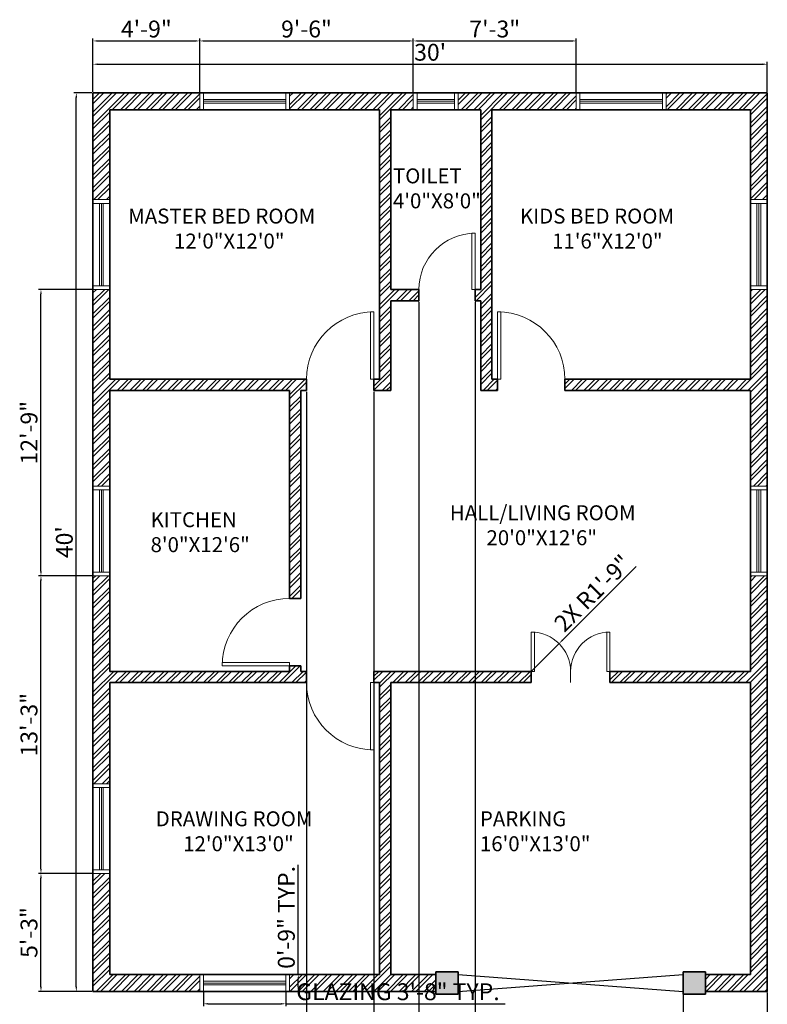
# Model space of a CAD drawing. Units: inches. Extents: x 2639 to 6021, y 292 to 2009.
# Tile 4 of 6: x 2697 to 3096, y 1243 to 1768. Entities that reach past the tile are written whole.
import ezdxf

# ---------------------------------------------------------------- set-up
doc = ezdxf.new("R2010")
doc.units = ezdxf.units.IN
for name, color, linetype, lineweight in [('A-ANNO-DIMS', 2, 'Continuous', 18), ('A-AREA-IDEN', 7, 'Continuous', 18), ('A-COLS', 7, 'Continuous', 35), ('A-DOOR', 3, 'Continuous', 20), ('A-DOOR-GATE', 3, 'Continuous', 25), ('A-GLAZ', 4, 'Continuous', 18), ('A-WALL', 7, 'Continuous', 35)]:
    doc.layers.add(name, color=color, linetype=linetype, lineweight=lineweight)
doc.layers.add('A-COLS-PATT', color=251, linetype='Continuous', lineweight=13, true_color=0x636466)
doc.layers.add('A-WALL-PATT', color=251, linetype='Continuous', lineweight=13, true_color=0x636466)
doc.styles.get("Standard").update_dxf_attribs({"font": 'arial.ttf'})
doc.dimstyles.new('ISO-25', dxfattribs={"dimtxt": 9, "dimasz": 2.5, "dimexe": 1.25, "dimexo": 0.625, "dimtad": 1, "dimdec": 1, "dimlunit": 3, "dimtxsty": 'Standard', "dimcen": 2.5, "dimadec": 0, "dimazin": 0, "dimtfac": 1, "dimtdec": 1, "dimtmove": 0, "dimatfit": 3, "dimfxl": 1, "dimarcsym": 0})

# ---------------------------------------------------------------- blocks, each defined once
blk = doc.blocks.new('*U2')
for p, q in [((0, 0), (0, -6)), ((30, 0), (30, -6))]:
    blk.add_line(p, q)
blk.add_lwpolyline([(0, 0), (0, 30), (1.75, 30), (1.75, 0)], close=True)
blk.add_arc((0, 0), 30, 0, 90)
blk = doc.blocks.new('*U3')
for p, q in [((0, 0), (0, -6)), ((36, 0), (36, -6))]:
    blk.add_line(p, q)
blk.add_lwpolyline([(0, 0), (0, 36), (1.75, 36), (1.75, 0)], close=True)
blk.add_arc((0, 0), 36, 0, 90)
blk = doc.blocks.new('1')
for p, q in [((0, 6), (0, 0)), ((21, 6), (21, 0)), ((21, 6), (21, 0)), ((42, 6), (42, 0))]:
    blk.add_line(p, q)
for points in [[(0, 6), (0, 27), (1.75, 27), (1.75, 6)], [(42, 6), (42, 27), (40.25, 27), (40.25, 6)]]:
    blk.add_lwpolyline(points, close=True)
for centre, start, end in [((0, 6), 0, 90), ((42, 6), 90, 180)]:
    blk.add_arc(centre, 21, start, end)
blk = doc.blocks.new('*D5')
at = {"layer": 'A-ANNO-DIMS', "color": 0, "lineweight": -2, "transparency": 16777216}
for p, q in [((2735.48, 1729.38), (2725.97, 1729.38)), ((2727.22, 1251.88), (2727.22, 1726.88)), ((2735.48, 1249.38), (2725.97, 1249.38))]:
    blk.add_line(p, q, dxfattribs=at)
at = {"layer": 'A-ANNO-DIMS', "color": 0, "transparency": 16777216}
for points in [[(2726.81, 1726.88), (2727.64, 1726.88), (2727.22, 1729.38)], [(2726.81, 1251.88), (2727.64, 1251.88), (2727.22, 1249.38)]]:
    blk.add_solid(points, dxfattribs=at)
at = {"layer": 'Defpoints', "color": 0, "transparency": 16777216}
for p in [(2727.22, 1729.38), (2736.11, 1729.38), (2736.11, 1249.38)]:
    blk.add_point(p, dxfattribs=at)
at = {"layer": 'A-ANNO-DIMS', "color": 0, "transparency": 16777216, "insert": (2722, 1489.38), "char_height": 9, "attachment_point": 5, "rotation": 90}
blk.add_mtext("40'", dxfattribs=at)
blk = doc.blocks.new('*D6')
at = {"layer": 'A-ANNO-DIMS', "color": 0, "lineweight": -2, "transparency": 16777216}
for p, q in [((2736.11, 1730.01), (2736.11, 1745.96)), ((2738.61, 1744.71), (3093.61, 1744.71)), ((3096.11, 1730.01), (3096.11, 1745.96))]:
    blk.add_line(p, q, dxfattribs=at)
at = {"layer": 'A-ANNO-DIMS', "color": 0, "transparency": 16777216}
for points in [[(2738.61, 1745.12), (2738.61, 1744.29), (2736.11, 1744.71)], [(3093.61, 1745.12), (3093.61, 1744.29), (3096.11, 1744.71)]]:
    blk.add_solid(points, dxfattribs=at)
at = {"layer": 'Defpoints', "color": 0, "transparency": 16777216}
for p in [(3096.11, 1744.71), (2736.11, 1729.38), (3096.11, 1729.38)]:
    blk.add_point(p, dxfattribs=at)
at = {"layer": 'A-ANNO-DIMS', "color": 0, "transparency": 16777216, "insert": (2916.11, 1749.93), "char_height": 9, "attachment_point": 5}
blk.add_mtext("30'", dxfattribs=at)
blk = doc.blocks.new('WINDOW-PLAN-48IN')
for p, q in [((0, 9), (0, 0)), ((0, 5.5), (44, 5.5)), ((44, 9), (44, 0)), ((0, 4.5), (44, 4.5)), ((0, 3.5), (44, 3.5))]:
    blk.add_line(p, q)
blk = doc.blocks.new('WINDOW-PLAN-24IN')
for p, q in [((0, 0), (0, 9)), ((0, 5.5), (20, 5.5)), ((20, 0), (20, 9)), ((0, 4.5), (20, 4.5)), ((0, 3.5), (20, 3.5))]:
    blk.add_line(p, q)
blk = doc.blocks.new('GATE-PLAN-10FT')
for p, q in [((0, 9), (120, 0)), ((0, 0), (120, 9))]:
    blk.add_line(p, q)
blk = doc.blocks.new('*D32')
at = {"layer": 'A-ANNO-DIMS', "color": 0, "lineweight": -2, "transparency": 16777216}
for p, q in [((2795.11, 1248.76), (2795.11, 1241.53)), ((2839.11, 1248.76), (2839.11, 1241.53)), ((2797.61, 1242.78), (2836.61, 1242.78)), ((2839.11, 1242.78), (2956.25, 1242.78))]:
    blk.add_line(p, q, dxfattribs=at)
at = {"layer": 'A-ANNO-DIMS', "color": 0, "transparency": 16777216}
for points in [[(2797.61, 1243.2), (2797.61, 1242.37), (2795.11, 1242.78)], [(2836.61, 1243.2), (2836.61, 1242.37), (2839.11, 1242.78)]]:
    blk.add_solid(points, dxfattribs=at)
at = {"layer": 'Defpoints', "color": 0, "transparency": 16777216}
for p in [(2795.11, 1249.38), (2839.11, 1249.38), (2839.11, 1242.78)]:
    blk.add_point(p, dxfattribs=at)
at = {"layer": 'A-ANNO-DIMS', "color": 0, "transparency": 16777216, "insert": (2898.93, 1248.07), "char_height": 9, "attachment_point": 5}
blk.add_mtext('GLAZING 3\'-8" TYP.', dxfattribs=at)
blk = doc.blocks.new('*D33')
at = {"layer": 'A-ANNO-DIMS', "color": 0, "lineweight": -2, "transparency": 16777216}
for p, q in [((2845.71, 1258.38), (2845.71, 1316.99)), ((2839.73, 1258.38), (2846.96, 1258.38)), ((2845.71, 1251.88), (2845.71, 1255.88)), ((2839.73, 1249.38), (2846.96, 1249.38))]:
    blk.add_line(p, q, dxfattribs=at)
at = {"layer": 'A-ANNO-DIMS', "color": 0, "transparency": 16777216}
for points in [[(2845.29, 1255.88), (2846.12, 1255.88), (2845.71, 1258.38)], [(2845.29, 1251.88), (2846.12, 1251.88), (2845.71, 1249.38)]]:
    blk.add_solid(points, dxfattribs=at)
at = {"layer": 'Defpoints', "color": 0, "transparency": 16777216}
for p in [(2839.11, 1258.38), (2845.71, 1258.38), (2839.11, 1249.38)]:
    blk.add_point(p, dxfattribs=at)
at = {"layer": 'A-ANNO-DIMS', "color": 0, "transparency": 16777216, "insert": (2840.49, 1288.94), "char_height": 9, "attachment_point": 5, "rotation": 90}
blk.add_mtext('0\'-9" TYP.', dxfattribs=at)
blk = doc.blocks.new('*D54')
at = {"layer": 'A-ANNO-DIMS', "color": 0, "lineweight": -2, "transparency": 16777216}
for p, q in [((2850.11, 1569.76), (2850.11, 1218.88)), ((2886.11, 1569.76), (2886.11, 1218.88)), ((2852.61, 1220.13), (2883.61, 1220.13))]:
    blk.add_line(p, q, dxfattribs=at)
at = {"layer": 'A-ANNO-DIMS', "color": 0, "transparency": 16777216}
for points in [[(2852.61, 1220.55), (2852.61, 1219.72), (2850.11, 1220.13)], [(2883.61, 1220.55), (2883.61, 1219.72), (2886.11, 1220.13)]]:
    blk.add_solid(points, dxfattribs=at)
at = {"layer": 'Defpoints', "color": 0, "transparency": 16777216}
for p in [(2850.11, 1570.38), (2886.11, 1570.38), (2886.11, 1220.13)]:
    blk.add_point(p, dxfattribs=at)
at = {"layer": 'A-ANNO-DIMS', "color": 0, "transparency": 16777216, "insert": (2868.11, 1225.36), "char_height": 9, "attachment_point": 5}
blk.add_mtext('3\'-0"', dxfattribs=at)
blk = doc.blocks.new('*D55')
at = {"layer": 'A-ANNO-DIMS', "color": 0, "lineweight": -2, "transparency": 16777216}
for p, q in [((2910.11, 1617.76), (2910.11, 1218.88)), ((2940.11, 1617.76), (2940.11, 1218.88)), ((2912.61, 1220.13), (2937.61, 1220.13))]:
    blk.add_line(p, q, dxfattribs=at)
at = {"layer": 'A-ANNO-DIMS', "color": 0, "transparency": 16777216}
for points in [[(2912.61, 1220.55), (2912.61, 1219.72), (2910.11, 1220.13)], [(2937.61, 1220.55), (2937.61, 1219.72), (2940.11, 1220.13)]]:
    blk.add_solid(points, dxfattribs=at)
at = {"layer": 'Defpoints', "color": 0, "transparency": 16777216}
for p in [(2910.11, 1618.38), (2940.11, 1618.38), (2940.11, 1220.13)]:
    blk.add_point(p, dxfattribs=at)
at = {"layer": 'A-ANNO-DIMS', "color": 0, "transparency": 16777216, "insert": (2925.11, 1225.35), "char_height": 9, "attachment_point": 5}
blk.add_mtext('2\'-6"', dxfattribs=at)
blk = doc.blocks.new('*D56')
at = {"layer": 'A-ANNO-DIMS', "color": 0, "lineweight": -2, "transparency": 16777216}
for p, q in [((2736.11, 1730.01), (2736.11, 1758.38)), ((2738.61, 1757.13), (2790.61, 1757.13)), ((2793.11, 1730.01), (2793.11, 1758.38))]:
    blk.add_line(p, q, dxfattribs=at)
at = {"layer": 'A-ANNO-DIMS', "color": 0, "transparency": 16777216}
for points in [[(2738.61, 1757.55), (2738.61, 1756.72), (2736.11, 1757.13)], [(2790.61, 1757.55), (2790.61, 1756.72), (2793.11, 1757.13)]]:
    blk.add_solid(points, dxfattribs=at)
at = {"layer": 'Defpoints', "color": 0, "transparency": 16777216}
for p in [(2793.11, 1757.13), (2736.11, 1729.38), (2793.11, 1729.38)]:
    blk.add_point(p, dxfattribs=at)
at = {"layer": 'A-ANNO-DIMS', "color": 0, "transparency": 16777216, "insert": (2764.61, 1762.35), "char_height": 9, "attachment_point": 5}
blk.add_mtext('4\'-9"', dxfattribs=at)
blk = doc.blocks.new('*D57')
at = {"layer": 'A-ANNO-DIMS', "color": 0, "lineweight": -2, "transparency": 16777216}
for p, q in [((2793.11, 1730.01), (2793.11, 1758.38)), ((2795.61, 1757.13), (2904.61, 1757.13)), ((2907.11, 1730.01), (2907.11, 1758.38))]:
    blk.add_line(p, q, dxfattribs=at)
at = {"layer": 'A-ANNO-DIMS', "color": 0, "transparency": 16777216}
for points in [[(2795.61, 1757.55), (2795.61, 1756.72), (2793.11, 1757.13)], [(2904.61, 1757.55), (2904.61, 1756.72), (2907.11, 1757.13)]]:
    blk.add_solid(points, dxfattribs=at)
at = {"layer": 'Defpoints', "color": 0, "transparency": 16777216}
for p in [(2907.11, 1757.13), (2793.11, 1729.38), (2907.11, 1729.38)]:
    blk.add_point(p, dxfattribs=at)
at = {"layer": 'A-ANNO-DIMS', "color": 0, "transparency": 16777216, "insert": (2850.11, 1762.35), "char_height": 9, "attachment_point": 5}
blk.add_mtext('9\'-6"', dxfattribs=at)
blk = doc.blocks.new('*D58')
at = {"layer": 'A-ANNO-DIMS', "color": 0, "lineweight": -2, "transparency": 16777216}
for p, q in [((2907.11, 1730.01), (2907.11, 1758.38)), ((2909.61, 1757.13), (2991.61, 1757.13)), ((2994.11, 1730.01), (2994.11, 1758.38))]:
    blk.add_line(p, q, dxfattribs=at)
at = {"layer": 'A-ANNO-DIMS', "color": 0, "transparency": 16777216}
for points in [[(2909.61, 1757.55), (2909.61, 1756.72), (2907.11, 1757.13)], [(2991.61, 1757.55), (2991.61, 1756.72), (2994.11, 1757.13)]]:
    blk.add_solid(points, dxfattribs=at)
at = {"layer": 'Defpoints', "color": 0, "transparency": 16777216}
for p in [(2994.11, 1757.13), (2907.11, 1729.38), (2994.11, 1729.38)]:
    blk.add_point(p, dxfattribs=at)
at = {"layer": 'A-ANNO-DIMS', "color": 0, "transparency": 16777216, "insert": (2950.61, 1762.36), "char_height": 9, "attachment_point": 5}
blk.add_mtext('7\'-3"', dxfattribs=at)
blk = doc.blocks.new('*D59')
at = {"layer": 'A-ANNO-DIMS', "color": 0, "lineweight": -2, "transparency": 16777216}
for p, q in [((3051.11, 1248.76), (3051.11, 1218.88)), ((3096.11, 1248.76), (3096.11, 1218.88)), ((3093.61, 1220.13), (3053.61, 1220.13))]:
    blk.add_line(p, q, dxfattribs=at)
at = {"layer": 'A-ANNO-DIMS', "color": 0, "transparency": 16777216}
for points in [[(3053.61, 1220.55), (3053.61, 1219.72), (3051.11, 1220.13)], [(3093.61, 1220.55), (3093.61, 1219.72), (3096.11, 1220.13)]]:
    blk.add_solid(points, dxfattribs=at)
at = {"layer": 'Defpoints', "color": 0, "transparency": 16777216}
for p in [(3051.11, 1249.38), (3096.11, 1249.38), (3051.11, 1220.13)]:
    blk.add_point(p, dxfattribs=at)
at = {"layer": 'A-ANNO-DIMS', "color": 0, "transparency": 16777216, "insert": (3073.61, 1225.36), "char_height": 9, "attachment_point": 5}
blk.add_mtext('3\'-9"', dxfattribs=at)
blk = doc.blocks.new('*D60')
at = {"layer": 'A-ANNO-DIMS', "color": 0, "lineweight": -2, "transparency": 16777216}
for p, q in [((2735.48, 1312.38), (2707.11, 1312.38)), ((2708.36, 1251.88), (2708.36, 1309.88)), ((2735.48, 1249.38), (2707.11, 1249.38))]:
    blk.add_line(p, q, dxfattribs=at)
at = {"layer": 'A-ANNO-DIMS', "color": 0, "transparency": 16777216}
for points in [[(2707.94, 1309.88), (2708.77, 1309.88), (2708.36, 1312.38)], [(2707.94, 1251.88), (2708.77, 1251.88), (2708.36, 1249.38)]]:
    blk.add_solid(points, dxfattribs=at)
at = {"layer": 'Defpoints', "color": 0, "transparency": 16777216}
for p in [(2708.36, 1312.38), (2736.11, 1312.38), (2736.11, 1249.38)]:
    blk.add_point(p, dxfattribs=at)
at = {"layer": 'A-ANNO-DIMS', "color": 0, "transparency": 16777216, "insert": (2703.13, 1280.88), "char_height": 9, "attachment_point": 5, "rotation": 90}
blk.add_mtext('5\'-3"', dxfattribs=at)
blk = doc.blocks.new('*D61')
at = {"layer": 'A-ANNO-DIMS', "color": 0, "lineweight": -2, "transparency": 16777216}
for p, q in [((2735.48, 1471.38), (2707.11, 1471.38)), ((2708.36, 1314.88), (2708.36, 1468.88)), ((2735.48, 1312.38), (2707.11, 1312.38))]:
    blk.add_line(p, q, dxfattribs=at)
at = {"layer": 'A-ANNO-DIMS', "color": 0, "transparency": 16777216}
for points in [[(2707.94, 1468.88), (2708.77, 1468.88), (2708.36, 1471.38)], [(2707.94, 1314.88), (2708.77, 1314.88), (2708.36, 1312.38)]]:
    blk.add_solid(points, dxfattribs=at)
at = {"layer": 'Defpoints', "color": 0, "transparency": 16777216}
for p in [(2708.36, 1471.38), (2736.11, 1471.38), (2736.11, 1312.38)]:
    blk.add_point(p, dxfattribs=at)
at = {"layer": 'A-ANNO-DIMS', "color": 0, "transparency": 16777216, "insert": (2703.13, 1391.88), "char_height": 9, "attachment_point": 5, "rotation": 90}
blk.add_mtext('13\'-3"', dxfattribs=at)
blk = doc.blocks.new('*D62')
at = {"layer": 'A-ANNO-DIMS', "color": 0, "lineweight": -2, "transparency": 16777216}
for p, q in [((2735.48, 1624.38), (2707.11, 1624.38)), ((2708.36, 1473.88), (2708.36, 1621.88)), ((2735.48, 1471.38), (2707.11, 1471.38))]:
    blk.add_line(p, q, dxfattribs=at)
at = {"layer": 'A-ANNO-DIMS', "color": 0, "transparency": 16777216}
for points in [[(2707.94, 1621.88), (2708.77, 1621.88), (2708.36, 1624.38)], [(2707.94, 1473.88), (2708.77, 1473.88), (2708.36, 1471.38)]]:
    blk.add_solid(points, dxfattribs=at)
at = {"layer": 'Defpoints', "color": 0, "transparency": 16777216}
for p in [(2708.36, 1624.38), (2736.11, 1624.38), (2736.11, 1471.38)]:
    blk.add_point(p, dxfattribs=at)
at = {"layer": 'A-ANNO-DIMS', "color": 0, "transparency": 16777216, "insert": (2703.14, 1547.88), "char_height": 9, "attachment_point": 5, "rotation": 90}
blk.add_mtext('12\'-9"', dxfattribs=at)
blk = doc.blocks.new('*D112')
at = {"layer": 'A-ANNO-DIMS', "color": 0, "lineweight": -2, "transparency": 16777216}
for p, q in [((3026.17, 1476.44), (2986.72, 1437)), ((2970.11, 1420.38), (2984.96, 1435.23))]:
    blk.add_line(p, q, dxfattribs=at)
at = {"layer": 'A-ANNO-DIMS', "color": 0, "transparency": 16777216}
blk.add_solid([(2986.43, 1437.3), (2987.02, 1436.71), (2984.96, 1435.23)], dxfattribs=at)
at = {"layer": 'Defpoints', "color": 0, "transparency": 16777216}
for p in [(2984.96, 1435.23), (2970.11, 1420.38)]:
    blk.add_point(p, dxfattribs=at)
at = {"layer": 'A-ANNO-DIMS', "color": 0, "transparency": 16777216, "insert": (3003.64, 1461.3), "char_height": 9, "attachment_point": 5, "rotation": 44.9996}
blk.add_mtext('2X R1\'-9"', dxfattribs=at)

msp = doc.modelspace()

# ---------------------------------------------------------------- hatches: boundary and pattern name
at = {"layer": 'A-COLS-PATT'}
h = msp.add_hatch(color=256, dxfattribs=at)
h.dxf.hatch_style = 1
h.paths.add_polyline_path([(2931.11, 1259.88), (2919.11, 1259.88), (2919.11, 1247.88), (2931.11, 1247.88)])
h.paths.add_polyline_path([(3063.11, 1259.88), (3051.11, 1259.88), (3051.11, 1247.88), (3063.11, 1247.88)])
at = {"layer": 'A-WALL-PATT'}
h = msp.add_hatch(dxfattribs=at)
h.set_pattern_fill('ANSI32', color=256, scale=0.5)
h.paths.add_polyline_path([(2793.11, 1729.38), (2736.11, 1729.38), (2736.11, 1672.38), (2745.11, 1672.38), (2745.11, 1720.38), (2793.11, 1720.38)])
h.paths.add_polyline_path([(2907.11, 1729.38), (2841.11, 1729.38), (2841.11, 1720.38), (2889.11, 1720.38), (2889.11, 1576.38), (2886.11, 1576.38), (2886.11, 1570.38), (2895.11, 1570.38), (2895.11, 1618.38), (2910.11, 1618.38), (2910.11, 1624.38), (2895.11, 1624.38), (2895.11, 1720.38), (2907.11, 1720.38)])
h.paths.add_polyline_path([(2994.11, 1729.38), (2931.11, 1729.38), (2931.11, 1720.38), (2943.11, 1720.38), (2943.11, 1624.38), (2940.11, 1624.38), (2940.11, 1618.38), (2943.11, 1618.38), (2943.11, 1570.38), (2952.11, 1570.38), (2952.11, 1576.38), (2949.11, 1576.38), (2949.11, 1720.38), (2994.11, 1720.38)])
h.paths.add_polyline_path([(3096.11, 1729.38), (3042.11, 1729.38), (3042.11, 1720.38), (3087.11, 1720.38), (3087.11, 1672.38), (3096.11, 1672.38)])
h.paths.add_polyline_path([(2745.11, 1624.38), (2736.11, 1624.38), (2736.11, 1519.38), (2745.11, 1519.38), (2745.11, 1570.38), (2841.11, 1570.38), (2841.11, 1459.38), (2847.11, 1459.38), (2847.11, 1570.38), (2850.11, 1570.38), (2850.11, 1576.38), (2745.11, 1576.38)])
h.paths.add_polyline_path([(3096.11, 1624.38), (3087.11, 1624.38), (3087.11, 1576.38), (2988.11, 1576.38), (2988.11, 1570.38), (3087.11, 1570.38), (3087.11, 1519.38), (3096.11, 1519.38)])
h.paths.add_polyline_path([(2970.11, 1420.38), (2886.11, 1420.38), (2886.11, 1414.38), (2889.11, 1414.38), (2889.11, 1258.38), (2841.11, 1258.38), (2841.11, 1249.38), (2919.11, 1249.38), (2919.11, 1258.38), (2895.11, 1258.38), (2895.11, 1414.38), (2970.11, 1414.38)])
h.paths.add_polyline_path([(3096.11, 1471.38), (3087.11, 1471.38), (3087.11, 1420.38), (3012.11, 1420.38), (3012.11, 1414.38), (3087.11, 1414.38), (3087.11, 1258.38), (3063.11, 1258.38), (3063.11, 1249.38), (3096.11, 1249.38)])
h.paths.add_polyline_path([(2850.11, 1420.38), (2847.11, 1420.38), (2847.11, 1423.37), (2841.11, 1423.37), (2841.11, 1420.38), (2745.11, 1420.38), (2745.11, 1471.38), (2736.11, 1471.38), (2736.11, 1360.38), (2745.11, 1360.38), (2745.11, 1414.38), (2850.11, 1414.38)])
h.paths.add_polyline_path([(2745.11, 1312.38), (2736.11, 1312.38), (2736.11, 1249.38), (2793.11, 1249.38), (2793.11, 1258.38), (2745.11, 1258.38)])

# ---------------------------------------------------------------- linework, layer by layer
at = {"layer": 'A-COLS'}
for p, q in [((2919.11, 1259.88), (2919.11, 1247.88)), ((2919.11, 1259.88), (2931.11, 1259.88)), ((2931.11, 1259.88), (2931.11, 1247.88)), ((3051.11, 1259.88), (3051.11, 1247.88)), ((3051.11, 1259.88), (3063.11, 1259.88)), ((3063.11, 1259.88), (3063.11, 1247.88))]:
    msp.add_line(p, q, dxfattribs=at)
for points in [[(2919.11, 1247.88), (2931.11, 1247.88)], [(3051.11, 1247.88), (3063.11, 1247.88)]]:
    msp.add_lwpolyline(points, dxfattribs=at)
at = {"layer": 'A-GLAZ'}
for p, q in [((2793.11, 1720.38), (2793.11, 1729.38)), ((2841.11, 1720.38), (2841.11, 1729.38)), ((2907.11, 1720.38), (2907.11, 1729.38)), ((2931.11, 1720.38), (2931.11, 1729.38)), ((2994.11, 1720.38), (2994.11, 1729.38)), ((3042.11, 1720.38), (3042.11, 1729.38)), ((2745.11, 1672.38), (2736.11, 1672.38)), ((3087.11, 1672.38), (3096.11, 1672.38)), ((2745.11, 1624.38), (2736.11, 1624.38)), ((3087.11, 1624.38), (3096.11, 1624.38)), ((2745.11, 1519.38), (2736.11, 1519.38)), ((3087.11, 1519.38), (3096.11, 1519.38)), ((2745.11, 1471.38), (2736.11, 1471.38)), ((3087.11, 1471.38), (3096.11, 1471.38)), ((2745.11, 1360.38), (2736.11, 1360.38)), ((2745.11, 1312.38), (2736.11, 1312.38)), ((2793.11, 1258.38), (2793.11, 1249.38)), ((2841.11, 1258.38), (2841.11, 1249.38))]:
    msp.add_line(p, q, dxfattribs=at)
at = {"layer": 'A-WALL'}
for p, q in [((2745.11, 1720.38), (2745.11, 1576.38)), ((2889.11, 1720.38), (2745.11, 1720.38)), ((2889.11, 1720.38), (2889.11, 1576.38)), ((2895.11, 1720.38), (2895.11, 1624.38)), ((2943.11, 1720.38), (2895.11, 1720.38)), ((2943.11, 1720.38), (2943.11, 1624.38)), ((3087.11, 1720.38), (2949.11, 1720.38)), ((2949.11, 1720.38), (2949.11, 1576.38)), ((3087.11, 1576.38), (3087.11, 1720.38)), ((2910.11, 1624.38), (2895.11, 1624.38)), ((2910.11, 1624.38), (2910.11, 1618.38)), ((2943.11, 1624.38), (2940.11, 1624.38)), ((2940.11, 1624.38), (2940.11, 1618.38)), ((2910.11, 1618.38), (2895.11, 1618.38)), ((2895.11, 1618.38), (2895.11, 1570.38)), ((2943.11, 1618.38), (2940.11, 1618.38)), ((2943.11, 1618.38), (2943.11, 1570.38)), ((2850.11, 1576.38), (2745.11, 1576.38)), ((2850.11, 1576.38), (2850.11, 1570.38)), ((2889.11, 1576.38), (2886.11, 1576.38)), ((2886.11, 1576.38), (2886.11, 1570.38)), ((2952.11, 1576.38), (2949.11, 1576.38)), ((2952.11, 1576.38), (2952.11, 1570.38)), ((3087.11, 1576.38), (2988.11, 1576.38)), ((2988.11, 1576.38), (2988.11, 1570.38)), ((2841.11, 1570.38), (2745.11, 1570.38)), ((2745.11, 1570.38), (2745.11, 1420.38)), ((2841.11, 1570.38), (2841.11, 1459.38)), ((2847.11, 1570.38), (2847.11, 1459.38)), ((2850.11, 1570.38), (2847.11, 1570.38)), ((2895.11, 1570.38), (2886.11, 1570.38)), ((2952.11, 1570.38), (2943.11, 1570.38)), ((3087.11, 1570.38), (2988.11, 1570.38)), ((3087.11, 1420.38), (3087.11, 1570.38)), ((2847.11, 1459.38), (2841.11, 1459.38)), ((2841.11, 1420.38), (2745.11, 1420.38)), ((2847.11, 1423.38), (2841.11, 1423.38)), ((2841.11, 1423.38), (2841.11, 1420.38)), ((2847.11, 1423.38), (2847.11, 1420.38)), ((2850.11, 1420.38), (2847.11, 1420.38)), ((2850.11, 1420.38), (2850.11, 1414.38)), ((2886.11, 1420.38), (2886.11, 1414.38)), ((2970.11, 1420.38), (2886.11, 1420.38)), ((2970.11, 1414.38), (2970.11, 1420.38)), ((3087.11, 1420.38), (3012.11, 1420.38)), ((3012.11, 1414.38), (3012.11, 1420.38)), ((2745.11, 1414.38), (2745.11, 1258.38)), ((2850.11, 1414.38), (2745.11, 1414.38)), ((2889.11, 1414.38), (2886.11, 1414.38)), ((2889.11, 1414.38), (2889.11, 1258.38)), ((2895.11, 1414.38), (2895.11, 1258.38)), ((2970.11, 1414.38), (2895.11, 1414.38)), ((3087.11, 1414.38), (3012.11, 1414.38)), ((3087.11, 1258.38), (3087.11, 1414.38)), ((2745.11, 1258.38), (2889.11, 1258.38)), ((2895.11, 1258.38), (2919.11, 1258.38)), ((3063.11, 1258.38), (3087.11, 1258.38))]:
    msp.add_line(p, q, dxfattribs=at)
msp.add_lwpolyline([(3063.11, 1249.38), (3096.11, 1249.38), (3096.11, 1729.38), (2736.11, 1729.38), (2736.11, 1249.38), (2919.11, 1249.38)], dxfattribs=at)

# ---------------------------------------------------------------- block references
at = {"layer": 'A-DOOR', "xscale": -1}
for name, p in [('*U2', (2940.11, 1624.38)), ('*U3', (2886.11, 1576.38))]:
    msp.add_blockref(name, p, dxfattribs=at)
at = {"layer": 'A-DOOR'}
for name, p in [('*U3', (2952.11, 1576.38)), ('1', (2970.11, 1414.38))]:
    msp.add_blockref(name, p, dxfattribs=at)
for p, rotation in [((2841.11, 1423.37), 90), ((2886.11, 1414.38), 180)]:
    msp.add_blockref('*U3', p, dxfattribs=dict(at, rotation=rotation))
at = {"layer": 'A-DOOR-GATE'}
msp.add_blockref('GATE-PLAN-10FT', (2931.11, 1249.38), dxfattribs=at)
at = {"layer": 'A-GLAZ'}
for p, rotation in [((2839.11, 1729.38), 180), ((3040.11, 1729.38), 180), ((2745.11, 1626.38), 89.99999999999967), ((3096.11, 1626.38), 89.99999999999967), ((2745.11, 1473.38), 89.99999999999991), ((3096.11, 1473.38), 89.99999999999841), ((2745.11, 1314.38), 89.99999999999955)]:
    msp.add_blockref('WINDOW-PLAN-48IN', p, dxfattribs=dict(at, rotation=rotation))
for name, p in [('WINDOW-PLAN-24IN', (2909.11, 1720.38)), ('WINDOW-PLAN-48IN', (2795.11, 1249.38))]:
    msp.add_blockref(name, p, dxfattribs=at)

# ---------------------------------------------------------------- texts
at = {"layer": 'A-AREA-IDEN', "char_height": 8, "attachment_point": 1}
for s, insert in [('{\\fTimes New Roman|b0|i0|c0|p18;TOILET\\P4\'0"X8\'0"}', (2896.27, 1689.05)), ('{\\fTimes New Roman|b0|i0|c0|p18;MASTER BED ROOM\\P          12\'0"X12\'0"}', (2754.92, 1667.58)), ('{\\fTimes New Roman|b0|i0|c0|p18;KIDS BED ROOM\\P       11\'6"X12\'0"}', (2964.09, 1667.58)), ('{\\fTimes New Roman|b0|i0|c0|p18;HALL/LIVING ROOM\\P        20\'0"X12\'6"}', (2926.63, 1509.09)), ('{\\fTimes New Roman|b0|i0|c0|p18;KITCHEN\\P8\'0"X12\'6"}', (2766.86, 1505.4)), ('{\\fTimes New Roman|b0|i0|c0|p18;DRAWING ROOM\\P      12\'0"X13\'0"}', (2769.61, 1345.62)), ('{\\fTimes New Roman|b0|i0|c0|p18;PARKING\\P16\'0"X13\'0"}', (2942.69, 1345.62))]:
    msp.add_mtext_dynamic_manual_height_columns(s, width=172.2916, gutter_width=12.5, heights=[0], dxfattribs=dict(at, insert=insert))

# ---------------------------------------------------------------- dimensions: what is measured, and where the dimension line sits
at = {"layer": 'A-ANNO-DIMS'}
for base, p1, p2, override, picture, middle in [((2793.11, 1757.13), (2736.11, 1729.38), (2793.11, 1729.38), {"dimdec": 1, "dimlfac": 1, "dimrnd": 0, "dimzin": 1, "dimdsep": 46, "dimlunit": 4, "dimfrac": 2}, '*D56', (2764.61, 1762.35)), ((2907.11, 1757.13), (2793.11, 1729.38), (2907.11, 1729.38), {"dimdec": 1, "dimlfac": 1, "dimrnd": 0, "dimzin": 1, "dimdsep": 46, "dimlunit": 4, "dimfrac": 2}, '*D57', (2850.11, 1762.35)), ((2994.11, 1757.13), (2907.11, 1729.38), (2994.11, 1729.38), {"dimdec": 1, "dimlfac": 1, "dimrnd": 0, "dimzin": 1, "dimdsep": 46, "dimlunit": 4, "dimfrac": 2}, '*D58', (2950.61, 1762.36)), ((3096.11, 1744.71), (2736.11, 1729.38), (3096.11, 1729.38), {"dimclrd": 0, "dimclre": 0, "dimclrt": 0}, '*D6', (2916.11, 1749.93)), ((2940.11, 1220.13), (2910.11, 1618.38), (2940.11, 1618.38), {"dimdec": 1, "dimlfac": 1, "dimrnd": 0, "dimzin": 1, "dimdsep": 46, "dimlunit": 4, "dimfrac": 2}, '*D55', (2925.11, 1225.35)), ((2886.11, 1220.13), (2850.11, 1570.38), (2886.11, 1570.38), {"dimdec": 1, "dimlfac": 1, "dimrnd": 0, "dimzin": 1, "dimdsep": 46, "dimlunit": 4, "dimfrac": 2}, '*D54', (2868.11, 1225.36)), ((3051.11, 1220.13), (3096.11, 1249.38), (3051.11, 1249.38), {"dimdec": 1, "dimlfac": 1, "dimrnd": 0, "dimzin": 1, "dimdsep": 46, "dimlunit": 4, "dimfrac": 2}, '*D59', (3073.61, 1225.36))]:
    dim = msp.add_linear_dim(base=base, p1=p1, p2=p2, dimstyle='ISO-25', override=override, dxfattribs=at)
    dim.commit()
    dim.dimension.update_dxf_attribs({"geometry": picture, "text_midpoint": middle})
for base, p1, p2, override, picture, middle in [((2727.22, 1729.38), (2736.11, 1249.38), (2736.11, 1729.38), {"dimclrd": 0, "dimclre": 0, "dimclrt": 0}, '*D5', (2722, 1489.38)), ((2708.36, 1624.38), (2736.11, 1471.38), (2736.11, 1624.38), {"dimdec": 1, "dimlfac": 1, "dimrnd": 0, "dimzin": 1, "dimdsep": 46, "dimlunit": 4, "dimfrac": 2}, '*D62', (2703.14, 1547.88)), ((2708.36, 1471.38), (2736.11, 1312.38), (2736.11, 1471.38), {"dimdec": 1, "dimlfac": 1, "dimrnd": 0, "dimzin": 1, "dimdsep": 46, "dimlunit": 4, "dimfrac": 2}, '*D61', (2703.13, 1391.88)), ((2708.36, 1312.38), (2736.11, 1249.38), (2736.11, 1312.38), {"dimdec": 1, "dimlfac": 1, "dimrnd": 0, "dimzin": 1, "dimdsep": 46, "dimlunit": 4, "dimfrac": 2}, '*D60', (2703.13, 1280.88))]:
    dim = msp.add_linear_dim(base=base, p1=p1, p2=p2, angle=90, dimstyle='ISO-25', override=override, dxfattribs=at)
    dim.commit()
    dim.dimension.update_dxf_attribs({"geometry": picture, "text_midpoint": middle})
dim = msp.add_radius_dim(center=(2970.11, 1420.38), mpoint=(2984.96, 1435.23), text='2X <>', dimstyle='ISO-25', override={"dimdec": 1, "dimlfac": 1, "dimrnd": 0, "dimzin": 1, "dimdsep": 46, "dimlunit": 4, "dimfrac": 2}, dxfattribs=at)
dim.commit()
dim.dimension.update_dxf_attribs({"geometry": '*D112', "text_midpoint": (3003.64, 1461.3)})
dim = msp.add_linear_dim(base=(2845.71, 1258.38), p1=(2839.11, 1249.38), p2=(2839.11, 1258.38), angle=90, text='<> TYP.', dimstyle='ISO-25', override={"dimdec": 1, "dimlfac": 1, "dimrnd": 0, "dimzin": 1, "dimdsep": 46, "dimlunit": 4, "dimfrac": 2}, dxfattribs=at)
dim.commit()
dim.dimension.update_dxf_attribs({"geometry": '*D33', "text_midpoint": (2840.49, 1288.94)})
dim = msp.add_linear_dim(base=(2839.11, 1242.78), p1=(2795.11, 1249.38), p2=(2839.11, 1249.38), text='GLAZING <> TYP.', dimstyle='ISO-25', override={"dimdec": 1, "dimlfac": 1, "dimrnd": 0, "dimzin": 1, "dimdsep": 46, "dimlunit": 4, "dimfrac": 2}, dxfattribs=at)
dim.commit()
dim.dimension.update_dxf_attribs({"geometry": '*D32', "text_midpoint": (2898.93, 1248.07)})

doc.saveas('drawing.dxf')
